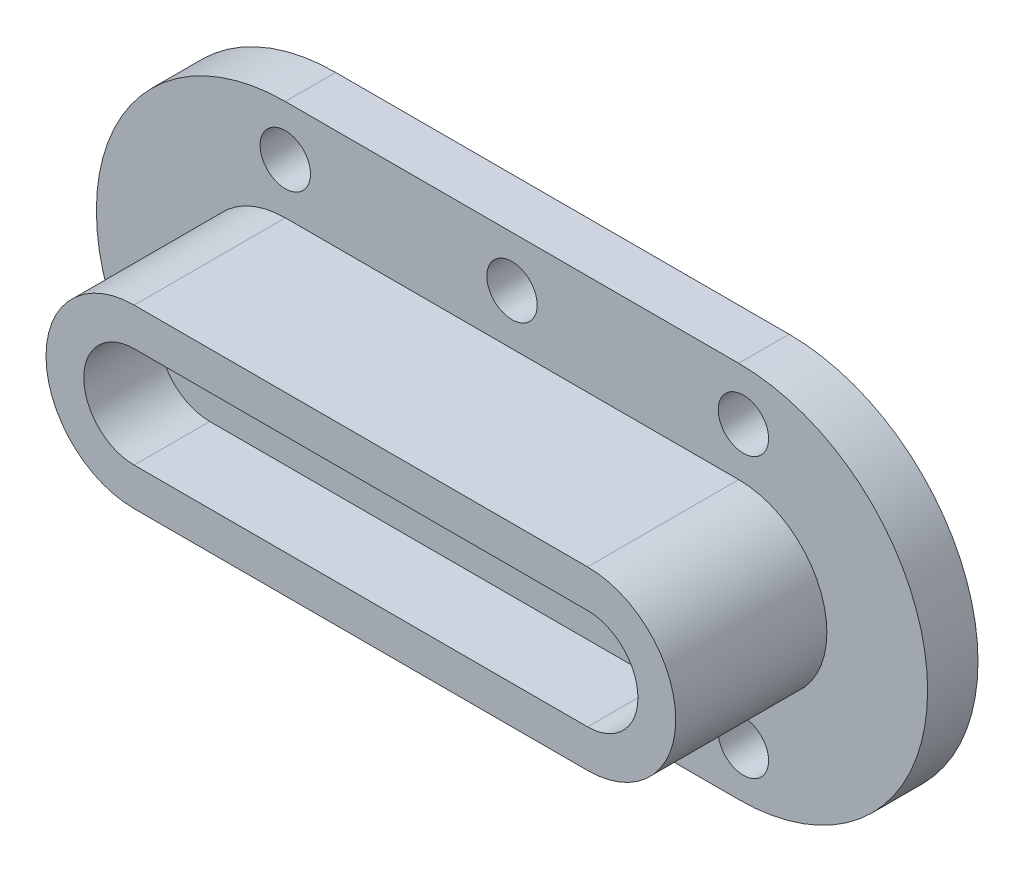
ISO-10303-21;
HEADER;
FILE_DESCRIPTION(('STEP AP214'),'2;1');
FILE_NAME('part.step','',(''),(''),'','','');
FILE_SCHEMA(('AUTOMOTIVE_DESIGN { 1 0 10303 214 1 1 1 1 }'));
ENDSEC;
DATA;
#1=APPLICATION_CONTEXT('core data for automotive mechanical design processes');
#2=APPLICATION_PROTOCOL_DEFINITION('international standard','automotive_design',2000,#1);
#3=PRODUCT_CONTEXT('',#1,'mechanical');
#4=PRODUCT('Part','Part','',(#3));
#5=PRODUCT_RELATED_PRODUCT_CATEGORY('part','',(#4));
#6=PRODUCT_DEFINITION_FORMATION('','',#4);
#7=PRODUCT_DEFINITION_CONTEXT('part definition',#1,'design');
#8=PRODUCT_DEFINITION('design','',#6,#7);
#9=PRODUCT_DEFINITION_SHAPE('','',#8);
#10=(LENGTH_UNIT() NAMED_UNIT(*) SI_UNIT(.MILLI.,.METRE.));
#11=(NAMED_UNIT(*) PLANE_ANGLE_UNIT() SI_UNIT($,.RADIAN.));
#12=(NAMED_UNIT(*) SI_UNIT($,.STERADIAN.) SOLID_ANGLE_UNIT());
#13=UNCERTAINTY_MEASURE_WITH_UNIT(LENGTH_MEASURE(1.E-05),#10,'distance_accuracy_value','');
#14=(GEOMETRIC_REPRESENTATION_CONTEXT(3) GLOBAL_UNCERTAINTY_ASSIGNED_CONTEXT((#13)) GLOBAL_UNIT_ASSIGNED_CONTEXT((#10,
#11,#12)) REPRESENTATION_CONTEXT('',''));
#15=CARTESIAN_POINT('',(0.,0.,0.));
#16=DIRECTION('',(0.,0.,1.));
#17=DIRECTION('',(1.,0.,0.));
#18=AXIS2_PLACEMENT_3D('',#15,#16,#17);
#19=CARTESIAN_POINT('',(0.,0.,20.));
#20=DIRECTION('',(0.,0.,-1.));
#21=DIRECTION('',(-1.,0.,0.));
#22=AXIS2_PLACEMENT_3D('',#19,#20,#21);
#23=CYLINDRICAL_SURFACE('',#22,75.);
#24=CARTESIAN_POINT('',(0.,0.,0.));
#25=DIRECTION('',(0.,0.,1.));
#26=DIRECTION('',(1.,0.,0.));
#27=AXIS2_PLACEMENT_3D('',#24,#25,#26);
#28=CIRCLE('',#27,75.);
#29=CARTESIAN_POINT('',(0.,75.,0.));
#30=VERTEX_POINT('',#29);
#31=CARTESIAN_POINT('',(0.,-75.,0.));
#32=VERTEX_POINT('',#31);
#33=EDGE_CURVE('E202',#30,#32,#28,.T.);
#34=ORIENTED_EDGE('',*,*,#33,.T.);
#35=DIRECTION('',(0.,0.,-1.));
#36=VECTOR('',#35,1.);
#37=CARTESIAN_POINT('',(0.,-75.,20.));
#38=LINE('',#37,#36);
#39=CARTESIAN_POINT('',(0.,-75.,20.));
#40=VERTEX_POINT('',#39);
#41=EDGE_CURVE('E11',#40,#32,#38,.T.);
#42=ORIENTED_EDGE('',*,*,#41,.F.);
#43=CARTESIAN_POINT('',(0.,0.,20.));
#44=DIRECTION('',(0.,0.,1.));
#45=DIRECTION('',(1.,0.,0.));
#46=AXIS2_PLACEMENT_3D('',#43,#44,#45);
#47=CIRCLE('',#46,75.);
#48=CARTESIAN_POINT('',(0.,75.,20.));
#49=VERTEX_POINT('',#48);
#50=EDGE_CURVE('E206',#49,#40,#47,.T.);
#51=ORIENTED_EDGE('',*,*,#50,.F.);
#52=DIRECTION('',(0.,0.,-1.));
#53=VECTOR('',#52,1.);
#54=CARTESIAN_POINT('',(0.,75.,20.));
#55=LINE('',#54,#53);
#56=EDGE_CURVE('E216',#49,#30,#55,.T.);
#57=ORIENTED_EDGE('',*,*,#56,.T.);
#58=EDGE_LOOP('',(#34,#42,#51,#57));
#59=FACE_BOUND('',#58,.T.);
#60=ADVANCED_FACE('F44',(#59),#23,.T.);
#61=CARTESIAN_POINT('',(0.,-75.,20.));
#62=DIRECTION('',(0.,1.,0.));
#63=DIRECTION('',(-1.,0.,0.));
#64=AXIS2_PLACEMENT_3D('',#61,#62,#63);
#65=PLANE('',#64);
#66=DIRECTION('',(1.,0.,0.));
#67=VECTOR('',#66,1.);
#68=CARTESIAN_POINT('',(0.,-75.,0.));
#69=LINE('',#68,#67);
#70=CARTESIAN_POINT('',(180.,-75.,0.));
#71=VERTEX_POINT('',#70);
#72=EDGE_CURVE('E218',#32,#71,#69,.T.);
#73=ORIENTED_EDGE('',*,*,#72,.T.);
#74=DIRECTION('',(0.,0.,-1.));
#75=VECTOR('',#74,1.);
#76=CARTESIAN_POINT('',(180.,-75.,20.));
#77=LINE('',#76,#75);
#78=CARTESIAN_POINT('',(180.,-75.,20.));
#79=VERTEX_POINT('',#78);
#80=EDGE_CURVE('E55',#79,#71,#77,.T.);
#81=ORIENTED_EDGE('',*,*,#80,.F.);
#82=DIRECTION('',(1.,0.,0.));
#83=VECTOR('',#82,1.);
#84=CARTESIAN_POINT('',(0.,-75.,20.));
#85=LINE('',#84,#83);
#86=EDGE_CURVE('E207',#40,#79,#85,.T.);
#87=ORIENTED_EDGE('',*,*,#86,.F.);
#88=ORIENTED_EDGE('',*,*,#41,.T.);
#89=EDGE_LOOP('',(#73,#81,#87,#88));
#90=FACE_BOUND('',#89,.T.);
#91=ADVANCED_FACE('F249',(#90),#65,.F.);
#92=CARTESIAN_POINT('',(180.,0.,20.));
#93=DIRECTION('',(0.,0.,-1.));
#94=DIRECTION('',(-1.,0.,0.));
#95=AXIS2_PLACEMENT_3D('',#92,#93,#94);
#96=CYLINDRICAL_SURFACE('',#95,75.);
#97=CARTESIAN_POINT('',(180.,0.,0.));
#98=DIRECTION('',(0.,0.,1.));
#99=DIRECTION('',(1.,0.,0.));
#100=AXIS2_PLACEMENT_3D('',#97,#98,#99);
#101=CIRCLE('',#100,75.);
#102=CARTESIAN_POINT('',(180.,75.,0.));
#103=VERTEX_POINT('',#102);
#104=EDGE_CURVE('E222',#71,#103,#101,.T.);
#105=ORIENTED_EDGE('',*,*,#104,.T.);
#106=DIRECTION('',(0.,0.,-1.));
#107=VECTOR('',#106,1.);
#108=CARTESIAN_POINT('',(180.,75.,20.));
#109=LINE('',#108,#107);
#110=CARTESIAN_POINT('',(180.,75.,20.));
#111=VERTEX_POINT('',#110);
#112=EDGE_CURVE('E227',#111,#103,#109,.T.);
#113=ORIENTED_EDGE('',*,*,#112,.F.);
#114=CARTESIAN_POINT('',(180.,0.,20.));
#115=DIRECTION('',(0.,0.,1.));
#116=DIRECTION('',(1.,0.,0.));
#117=AXIS2_PLACEMENT_3D('',#114,#115,#116);
#118=CIRCLE('',#117,75.);
#119=EDGE_CURVE('E215',#79,#111,#118,.T.);
#120=ORIENTED_EDGE('',*,*,#119,.F.);
#121=ORIENTED_EDGE('',*,*,#80,.T.);
#122=EDGE_LOOP('',(#105,#113,#120,#121));
#123=FACE_BOUND('',#122,.T.);
#124=ADVANCED_FACE('F231',(#123),#96,.T.);
#125=CARTESIAN_POINT('',(0.,75.,20.));
#126=DIRECTION('',(0.,-1.,0.));
#127=DIRECTION('',(1.,0.,0.));
#128=AXIS2_PLACEMENT_3D('',#125,#126,#127);
#129=PLANE('',#128);
#130=DIRECTION('',(-1.,0.,0.));
#131=VECTOR('',#130,1.);
#132=CARTESIAN_POINT('',(0.,75.,0.));
#133=LINE('',#132,#131);
#134=EDGE_CURVE('E209',#103,#30,#133,.T.);
#135=ORIENTED_EDGE('',*,*,#134,.T.);
#136=ORIENTED_EDGE('',*,*,#56,.F.);
#137=DIRECTION('',(-1.,0.,0.));
#138=VECTOR('',#137,1.);
#139=CARTESIAN_POINT('',(0.,75.,20.));
#140=LINE('',#139,#138);
#141=EDGE_CURVE('E212',#111,#49,#140,.T.);
#142=ORIENTED_EDGE('',*,*,#141,.F.);
#143=ORIENTED_EDGE('',*,*,#112,.T.);
#144=EDGE_LOOP('',(#135,#136,#142,#143));
#145=FACE_BOUND('',#144,.T.);
#146=ADVANCED_FACE('F245',(#145),#129,.F.);
#147=CARTESIAN_POINT('',(0.,0.,20.));
#148=DIRECTION('',(0.,0.,1.));
#149=DIRECTION('',(1.,0.,0.));
#150=AXIS2_PLACEMENT_3D('',#147,#148,#149);
#151=PLANE('',#150);
#152=CARTESIAN_POINT('',(181.871324801107,55.,20.));
#153=DIRECTION('',(0.,0.,1.));
#154=DIRECTION('',(1.,0.,0.));
#155=AXIS2_PLACEMENT_3D('',#152,#153,#154);
#156=CIRCLE('',#155,9.99999999999998);
#157=CARTESIAN_POINT('',(191.871324801107,55.,20.));
#158=VERTEX_POINT('',#157);
#159=EDGE_CURVE('E353',#158,#158,#156,.T.);
#160=ORIENTED_EDGE('',*,*,#159,.F.);
#161=EDGE_LOOP('',(#160));
#162=FACE_BOUND('',#161,.T.);
#163=CARTESIAN_POINT('',(181.871324801107,-55.7131327107115,20.));
#164=DIRECTION('',(0.,0.,1.));
#165=DIRECTION('',(1.,0.,0.));
#166=AXIS2_PLACEMENT_3D('',#163,#164,#165);
#167=CIRCLE('',#166,10.);
#168=CARTESIAN_POINT('',(191.871324801107,-55.7131327107115,20.));
#169=VERTEX_POINT('',#168);
#170=EDGE_CURVE('E359',#169,#169,#167,.T.);
#171=ORIENTED_EDGE('',*,*,#170,.F.);
#172=EDGE_LOOP('',(#171));
#173=FACE_BOUND('',#172,.T.);
#174=CARTESIAN_POINT('',(0.,-55.7131327107115,20.));
#175=DIRECTION('',(0.,0.,1.));
#176=DIRECTION('',(1.,0.,0.));
#177=AXIS2_PLACEMENT_3D('',#174,#175,#176);
#178=CIRCLE('',#177,10.);
#179=CARTESIAN_POINT('',(10.,-55.7131327107115,20.));
#180=VERTEX_POINT('',#179);
#181=EDGE_CURVE('E364',#180,#180,#178,.T.);
#182=ORIENTED_EDGE('',*,*,#181,.F.);
#183=EDGE_LOOP('',(#182));
#184=FACE_BOUND('',#183,.T.);
#185=CARTESIAN_POINT('',(90.,55.,20.));
#186=DIRECTION('',(0.,0.,1.));
#187=DIRECTION('',(1.,0.,0.));
#188=AXIS2_PLACEMENT_3D('',#185,#186,#187);
#189=CIRCLE('',#188,10.);
#190=CARTESIAN_POINT('',(100.,55.,20.));
#191=VERTEX_POINT('',#190);
#192=EDGE_CURVE('E347',#191,#191,#189,.T.);
#193=ORIENTED_EDGE('',*,*,#192,.F.);
#194=EDGE_LOOP('',(#193));
#195=FACE_BOUND('',#194,.T.);
#196=CARTESIAN_POINT('',(90.,-55.7131327107115,20.));
#197=DIRECTION('',(0.,0.,1.));
#198=DIRECTION('',(1.,0.,0.));
#199=AXIS2_PLACEMENT_3D('',#196,#197,#198);
#200=CIRCLE('',#199,9.99999999999999);
#201=CARTESIAN_POINT('',(100.,-55.7131327107115,20.));
#202=VERTEX_POINT('',#201);
#203=EDGE_CURVE('E341',#202,#202,#200,.T.);
#204=ORIENTED_EDGE('',*,*,#203,.F.);
#205=EDGE_LOOP('',(#204));
#206=FACE_BOUND('',#205,.T.);
#207=CARTESIAN_POINT('',(0.,55.,20.));
#208=DIRECTION('',(0.,0.,1.));
#209=DIRECTION('',(1.,0.,0.));
#210=AXIS2_PLACEMENT_3D('',#207,#208,#209);
#211=CIRCLE('',#210,10.);
#212=CARTESIAN_POINT('',(10.,55.,20.));
#213=VERTEX_POINT('',#212);
#214=EDGE_CURVE('E355',#213,#213,#211,.T.);
#215=ORIENTED_EDGE('',*,*,#214,.F.);
#216=EDGE_LOOP('',(#215));
#217=FACE_BOUND('',#216,.T.);
#218=CARTESIAN_POINT('',(0.,0.,20.));
#219=DIRECTION('',(0.,0.,1.));
#220=DIRECTION('',(1.,0.,0.));
#221=AXIS2_PLACEMENT_3D('',#218,#219,#220);
#222=CIRCLE('',#221,35.);
#223=CARTESIAN_POINT('',(0.,35.,20.));
#224=VERTEX_POINT('',#223);
#225=CARTESIAN_POINT('',(0.,-35.,20.));
#226=VERTEX_POINT('',#225);
#227=EDGE_CURVE('E70',#224,#226,#222,.T.);
#228=ORIENTED_EDGE('',*,*,#227,.F.);
#229=DIRECTION('',(-1.,0.,0.));
#230=VECTOR('',#229,1.);
#231=CARTESIAN_POINT('',(0.,35.,20.));
#232=LINE('',#231,#230);
#233=CARTESIAN_POINT('',(180.,35.,20.));
#234=VERTEX_POINT('',#233);
#235=EDGE_CURVE('E179',#234,#224,#232,.T.);
#236=ORIENTED_EDGE('',*,*,#235,.F.);
#237=CARTESIAN_POINT('',(180.,0.,20.));
#238=DIRECTION('',(0.,0.,1.));
#239=DIRECTION('',(1.,0.,0.));
#240=AXIS2_PLACEMENT_3D('',#237,#238,#239);
#241=CIRCLE('',#240,35.);
#242=CARTESIAN_POINT('',(180.,-35.,20.));
#243=VERTEX_POINT('',#242);
#244=EDGE_CURVE('E186',#243,#234,#241,.T.);
#245=ORIENTED_EDGE('',*,*,#244,.F.);
#246=DIRECTION('',(1.,0.,0.));
#247=VECTOR('',#246,1.);
#248=CARTESIAN_POINT('',(0.,-35.,20.));
#249=LINE('',#248,#247);
#250=EDGE_CURVE('E190',#226,#243,#249,.T.);
#251=ORIENTED_EDGE('',*,*,#250,.F.);
#252=EDGE_LOOP('',(#228,#236,#245,#251));
#253=FACE_BOUND('',#252,.T.);
#254=ORIENTED_EDGE('',*,*,#50,.T.);
#255=ORIENTED_EDGE('',*,*,#86,.T.);
#256=ORIENTED_EDGE('',*,*,#119,.T.);
#257=ORIENTED_EDGE('',*,*,#141,.T.);
#258=EDGE_LOOP('',(#254,#255,#256,#257));
#259=FACE_BOUND('',#258,.T.);
#260=ADVANCED_FACE('F246',(#162,#173,#184,#195,#206,#217,#253,#259),#151,.T.);
#261=CARTESIAN_POINT('',(0.,0.,0.));
#262=DIRECTION('',(0.,0.,1.));
#263=DIRECTION('',(1.,0.,0.));
#264=AXIS2_PLACEMENT_3D('',#261,#262,#263);
#265=PLANE('',#264);
#266=CARTESIAN_POINT('',(181.871324801107,55.,0.));
#267=DIRECTION('',(0.,0.,1.));
#268=DIRECTION('',(1.,0.,0.));
#269=AXIS2_PLACEMENT_3D('',#266,#267,#268);
#270=CIRCLE('',#269,9.99999999999998);
#271=CARTESIAN_POINT('',(191.871324801107,55.,0.));
#272=VERTEX_POINT('',#271);
#273=EDGE_CURVE('E349',#272,#272,#270,.T.);
#274=ORIENTED_EDGE('',*,*,#273,.T.);
#275=EDGE_LOOP('',(#274));
#276=FACE_BOUND('',#275,.T.);
#277=CARTESIAN_POINT('',(181.871324801107,-55.7131327107115,0.));
#278=DIRECTION('',(0.,0.,1.));
#279=DIRECTION('',(1.,0.,0.));
#280=AXIS2_PLACEMENT_3D('',#277,#278,#279);
#281=CIRCLE('',#280,10.);
#282=CARTESIAN_POINT('',(191.871324801107,-55.7131327107115,0.));
#283=VERTEX_POINT('',#282);
#284=EDGE_CURVE('E358',#283,#283,#281,.T.);
#285=ORIENTED_EDGE('',*,*,#284,.T.);
#286=EDGE_LOOP('',(#285));
#287=FACE_BOUND('',#286,.T.);
#288=CARTESIAN_POINT('',(0.,-55.7131327107115,0.));
#289=DIRECTION('',(0.,0.,1.));
#290=DIRECTION('',(1.,0.,0.));
#291=AXIS2_PLACEMENT_3D('',#288,#289,#290);
#292=CIRCLE('',#291,10.);
#293=CARTESIAN_POINT('',(10.,-55.7131327107115,0.));
#294=VERTEX_POINT('',#293);
#295=EDGE_CURVE('E362',#294,#294,#292,.T.);
#296=ORIENTED_EDGE('',*,*,#295,.T.);
#297=EDGE_LOOP('',(#296));
#298=FACE_BOUND('',#297,.T.);
#299=CARTESIAN_POINT('',(90.,55.,0.));
#300=DIRECTION('',(0.,0.,1.));
#301=DIRECTION('',(1.,0.,0.));
#302=AXIS2_PLACEMENT_3D('',#299,#300,#301);
#303=CIRCLE('',#302,10.);
#304=CARTESIAN_POINT('',(100.,55.,0.));
#305=VERTEX_POINT('',#304);
#306=EDGE_CURVE('E366',#305,#305,#303,.T.);
#307=ORIENTED_EDGE('',*,*,#306,.T.);
#308=EDGE_LOOP('',(#307));
#309=FACE_BOUND('',#308,.T.);
#310=CARTESIAN_POINT('',(90.,-55.7131327107115,0.));
#311=DIRECTION('',(0.,0.,1.));
#312=DIRECTION('',(1.,0.,0.));
#313=AXIS2_PLACEMENT_3D('',#310,#311,#312);
#314=CIRCLE('',#313,9.99999999999999);
#315=CARTESIAN_POINT('',(100.,-55.7131327107115,0.));
#316=VERTEX_POINT('',#315);
#317=EDGE_CURVE('E336',#316,#316,#314,.T.);
#318=ORIENTED_EDGE('',*,*,#317,.T.);
#319=EDGE_LOOP('',(#318));
#320=FACE_BOUND('',#319,.T.);
#321=CARTESIAN_POINT('',(0.,55.,0.));
#322=DIRECTION('',(0.,0.,1.));
#323=DIRECTION('',(1.,0.,0.));
#324=AXIS2_PLACEMENT_3D('',#321,#322,#323);
#325=CIRCLE('',#324,10.);
#326=CARTESIAN_POINT('',(10.,55.,0.));
#327=VERTEX_POINT('',#326);
#328=EDGE_CURVE('E373',#327,#327,#325,.T.);
#329=ORIENTED_EDGE('',*,*,#328,.T.);
#330=EDGE_LOOP('',(#329));
#331=FACE_BOUND('',#330,.T.);
#332=CARTESIAN_POINT('',(0.,0.,0.));
#333=DIRECTION('',(0.,0.,1.));
#334=DIRECTION('',(1.,0.,0.));
#335=AXIS2_PLACEMENT_3D('',#332,#333,#334);
#336=CIRCLE('',#335,7.5);
#337=CARTESIAN_POINT('',(7.5,0.,0.));
#338=VERTEX_POINT('',#337);
#339=EDGE_CURVE('E167',#338,#338,#336,.T.);
#340=ORIENTED_EDGE('',*,*,#339,.T.);
#341=EDGE_LOOP('',(#340));
#342=FACE_BOUND('',#341,.T.);
#343=CARTESIAN_POINT('',(180.,0.,0.));
#344=DIRECTION('',(0.,0.,1.));
#345=DIRECTION('',(1.,0.,0.));
#346=AXIS2_PLACEMENT_3D('',#343,#344,#345);
#347=CIRCLE('',#346,7.50000000000001);
#348=CARTESIAN_POINT('',(187.5,0.,0.));
#349=VERTEX_POINT('',#348);
#350=EDGE_CURVE('E382',#349,#349,#347,.T.);
#351=ORIENTED_EDGE('',*,*,#350,.T.);
#352=EDGE_LOOP('',(#351));
#353=FACE_BOUND('',#352,.T.);
#354=CARTESIAN_POINT('',(90.,0.,0.));
#355=DIRECTION('',(0.,0.,1.));
#356=DIRECTION('',(1.,0.,0.));
#357=AXIS2_PLACEMENT_3D('',#354,#355,#356);
#358=CIRCLE('',#357,7.5);
#359=CARTESIAN_POINT('',(97.5,0.,0.));
#360=VERTEX_POINT('',#359);
#361=EDGE_CURVE('E389',#360,#360,#358,.T.);
#362=ORIENTED_EDGE('',*,*,#361,.T.);
#363=EDGE_LOOP('',(#362));
#364=FACE_BOUND('',#363,.T.);
#365=ORIENTED_EDGE('',*,*,#33,.F.);
#366=ORIENTED_EDGE('',*,*,#134,.F.);
#367=ORIENTED_EDGE('',*,*,#104,.F.);
#368=ORIENTED_EDGE('',*,*,#72,.F.);
#369=EDGE_LOOP('',(#365,#366,#367,#368));
#370=FACE_BOUND('',#369,.T.);
#371=ADVANCED_FACE('F239',(#276,#287,#298,#309,#320,#331,#342,#353,#364,#370),#265,.F.);
#372=CARTESIAN_POINT('',(0.,0.,80.));
#373=DIRECTION('',(0.,0.,-1.));
#374=DIRECTION('',(-1.,0.,0.));
#375=AXIS2_PLACEMENT_3D('',#372,#373,#374);
#376=CYLINDRICAL_SURFACE('',#375,35.);
#377=ORIENTED_EDGE('',*,*,#227,.T.);
#378=DIRECTION('',(0.,0.,-1.));
#379=VECTOR('',#378,1.);
#380=CARTESIAN_POINT('',(0.,-35.,80.));
#381=LINE('',#380,#379);
#382=CARTESIAN_POINT('',(0.,-35.,80.));
#383=VERTEX_POINT('',#382);
#384=EDGE_CURVE('E205',#383,#226,#381,.T.);
#385=ORIENTED_EDGE('',*,*,#384,.F.);
#386=CARTESIAN_POINT('',(0.,0.,80.));
#387=DIRECTION('',(0.,0.,1.));
#388=DIRECTION('',(1.,0.,0.));
#389=AXIS2_PLACEMENT_3D('',#386,#387,#388);
#390=CIRCLE('',#389,35.);
#391=CARTESIAN_POINT('',(0.,35.,80.));
#392=VERTEX_POINT('',#391);
#393=EDGE_CURVE('E171',#392,#383,#390,.T.);
#394=ORIENTED_EDGE('',*,*,#393,.F.);
#395=DIRECTION('',(0.,0.,-1.));
#396=VECTOR('',#395,1.);
#397=CARTESIAN_POINT('',(0.,35.,80.));
#398=LINE('',#397,#396);
#399=EDGE_CURVE('E183',#392,#224,#398,.T.);
#400=ORIENTED_EDGE('',*,*,#399,.T.);
#401=EDGE_LOOP('',(#377,#385,#394,#400));
#402=FACE_BOUND('',#401,.T.);
#403=ADVANCED_FACE('F261',(#402),#376,.T.);
#404=CARTESIAN_POINT('',(0.,-35.,80.));
#405=DIRECTION('',(0.,1.,0.));
#406=DIRECTION('',(0.,0.,1.));
#407=AXIS2_PLACEMENT_3D('',#404,#405,#406);
#408=PLANE('',#407);
#409=ORIENTED_EDGE('',*,*,#250,.T.);
#410=DIRECTION('',(0.,0.,-1.));
#411=VECTOR('',#410,1.);
#412=CARTESIAN_POINT('',(180.,-35.,80.));
#413=LINE('',#412,#411);
#414=CARTESIAN_POINT('',(180.,-35.,80.));
#415=VERTEX_POINT('',#414);
#416=EDGE_CURVE('E200',#415,#243,#413,.T.);
#417=ORIENTED_EDGE('',*,*,#416,.F.);
#418=DIRECTION('',(1.,0.,0.));
#419=VECTOR('',#418,1.);
#420=CARTESIAN_POINT('',(0.,-35.,80.));
#421=LINE('',#420,#419);
#422=EDGE_CURVE('E176',#383,#415,#421,.T.);
#423=ORIENTED_EDGE('',*,*,#422,.F.);
#424=ORIENTED_EDGE('',*,*,#384,.T.);
#425=EDGE_LOOP('',(#409,#417,#423,#424));
#426=FACE_BOUND('',#425,.T.);
#427=ADVANCED_FACE('F268',(#426),#408,.F.);
#428=CARTESIAN_POINT('',(180.,0.,80.));
#429=DIRECTION('',(0.,0.,-1.));
#430=DIRECTION('',(-1.,0.,0.));
#431=AXIS2_PLACEMENT_3D('',#428,#429,#430);
#432=CYLINDRICAL_SURFACE('',#431,35.);
#433=ORIENTED_EDGE('',*,*,#244,.T.);
#434=DIRECTION('',(0.,0.,-1.));
#435=VECTOR('',#434,1.);
#436=CARTESIAN_POINT('',(180.,35.,80.));
#437=LINE('',#436,#435);
#438=CARTESIAN_POINT('',(180.,35.,80.));
#439=VERTEX_POINT('',#438);
#440=EDGE_CURVE('E198',#439,#234,#437,.T.);
#441=ORIENTED_EDGE('',*,*,#440,.F.);
#442=CARTESIAN_POINT('',(180.,0.,80.));
#443=DIRECTION('',(0.,0.,1.));
#444=DIRECTION('',(1.,0.,0.));
#445=AXIS2_PLACEMENT_3D('',#442,#443,#444);
#446=CIRCLE('',#445,35.);
#447=EDGE_CURVE('E182',#415,#439,#446,.T.);
#448=ORIENTED_EDGE('',*,*,#447,.F.);
#449=ORIENTED_EDGE('',*,*,#416,.T.);
#450=EDGE_LOOP('',(#433,#441,#448,#449));
#451=FACE_BOUND('',#450,.T.);
#452=ADVANCED_FACE('F275',(#451),#432,.T.);
#453=CARTESIAN_POINT('',(0.,35.,80.));
#454=DIRECTION('',(0.,-1.,0.));
#455=DIRECTION('',(0.,0.,-1.));
#456=AXIS2_PLACEMENT_3D('',#453,#454,#455);
#457=PLANE('',#456);
#458=ORIENTED_EDGE('',*,*,#235,.T.);
#459=ORIENTED_EDGE('',*,*,#399,.F.);
#460=DIRECTION('',(-1.,0.,0.));
#461=VECTOR('',#460,1.);
#462=CARTESIAN_POINT('',(0.,35.,80.));
#463=LINE('',#462,#461);
#464=EDGE_CURVE('E181',#439,#392,#463,.T.);
#465=ORIENTED_EDGE('',*,*,#464,.F.);
#466=ORIENTED_EDGE('',*,*,#440,.T.);
#467=EDGE_LOOP('',(#458,#459,#465,#466));
#468=FACE_BOUND('',#467,.T.);
#469=ADVANCED_FACE('F277',(#468),#457,.F.);
#470=CARTESIAN_POINT('',(0.,0.,80.));
#471=DIRECTION('',(0.,0.,1.));
#472=DIRECTION('',(1.,0.,0.));
#473=AXIS2_PLACEMENT_3D('',#470,#471,#472);
#474=PLANE('',#473);
#475=CARTESIAN_POINT('',(0.,0.,80.));
#476=DIRECTION('',(0.,0.,1.));
#477=DIRECTION('',(1.,0.,0.));
#478=AXIS2_PLACEMENT_3D('',#475,#476,#477);
#479=CIRCLE('',#478,20.);
#480=CARTESIAN_POINT('',(0.,20.,80.));
#481=VERTEX_POINT('',#480);
#482=CARTESIAN_POINT('',(0.,-20.,80.));
#483=VERTEX_POINT('',#482);
#484=EDGE_CURVE('E56',#481,#483,#479,.T.);
#485=ORIENTED_EDGE('',*,*,#484,.F.);
#486=DIRECTION('',(-1.,0.,0.));
#487=VECTOR('',#486,1.);
#488=CARTESIAN_POINT('',(0.,20.,80.));
#489=LINE('',#488,#487);
#490=CARTESIAN_POINT('',(180.,20.,80.));
#491=VERTEX_POINT('',#490);
#492=EDGE_CURVE('E153',#491,#481,#489,.T.);
#493=ORIENTED_EDGE('',*,*,#492,.F.);
#494=CARTESIAN_POINT('',(180.,0.,80.));
#495=DIRECTION('',(0.,0.,1.));
#496=DIRECTION('',(1.,0.,0.));
#497=AXIS2_PLACEMENT_3D('',#494,#495,#496);
#498=CIRCLE('',#497,20.);
#499=CARTESIAN_POINT('',(180.,-20.,80.));
#500=VERTEX_POINT('',#499);
#501=EDGE_CURVE('E156',#500,#491,#498,.T.);
#502=ORIENTED_EDGE('',*,*,#501,.F.);
#503=DIRECTION('',(1.,0.,0.));
#504=VECTOR('',#503,1.);
#505=CARTESIAN_POINT('',(0.,-20.,80.));
#506=LINE('',#505,#504);
#507=EDGE_CURVE('E164',#483,#500,#506,.T.);
#508=ORIENTED_EDGE('',*,*,#507,.F.);
#509=EDGE_LOOP('',(#485,#493,#502,#508));
#510=FACE_BOUND('',#509,.T.);
#511=ORIENTED_EDGE('',*,*,#393,.T.);
#512=ORIENTED_EDGE('',*,*,#422,.T.);
#513=ORIENTED_EDGE('',*,*,#447,.T.);
#514=ORIENTED_EDGE('',*,*,#464,.T.);
#515=EDGE_LOOP('',(#511,#512,#513,#514));
#516=FACE_BOUND('',#515,.T.);
#517=ADVANCED_FACE('F278',(#510,#516),#474,.T.);
#518=CARTESIAN_POINT('',(0.,0.,50.));
#519=DIRECTION('',(0.,0.,1.));
#520=DIRECTION('',(1.,0.,0.));
#521=AXIS2_PLACEMENT_3D('',#518,#519,#520);
#522=CYLINDRICAL_SURFACE('',#521,20.);
#523=ORIENTED_EDGE('',*,*,#484,.T.);
#524=DIRECTION('',(0.,0.,1.));
#525=VECTOR('',#524,1.);
#526=CARTESIAN_POINT('',(0.,-20.,50.));
#527=LINE('',#526,#525);
#528=CARTESIAN_POINT('',(0.,-20.,50.));
#529=VERTEX_POINT('',#528);
#530=EDGE_CURVE('E132',#529,#483,#527,.T.);
#531=ORIENTED_EDGE('',*,*,#530,.F.);
#532=CARTESIAN_POINT('',(0.,0.,50.));
#533=DIRECTION('',(0.,0.,1.));
#534=DIRECTION('',(1.,0.,0.));
#535=AXIS2_PLACEMENT_3D('',#532,#533,#534);
#536=CIRCLE('',#535,20.);
#537=CARTESIAN_POINT('',(0.,20.,50.));
#538=VERTEX_POINT('',#537);
#539=EDGE_CURVE('E131',#538,#529,#536,.T.);
#540=ORIENTED_EDGE('',*,*,#539,.F.);
#541=DIRECTION('',(0.,0.,1.));
#542=VECTOR('',#541,1.);
#543=CARTESIAN_POINT('',(0.,20.,50.));
#544=LINE('',#543,#542);
#545=EDGE_CURVE('E168',#538,#481,#544,.T.);
#546=ORIENTED_EDGE('',*,*,#545,.T.);
#547=EDGE_LOOP('',(#523,#531,#540,#546));
#548=FACE_BOUND('',#547,.T.);
#549=ADVANCED_FACE('F133',(#548),#522,.F.);
#550=CARTESIAN_POINT('',(0.,20.,50.));
#551=DIRECTION('',(0.,1.,0.));
#552=DIRECTION('',(-1.,0.,0.));
#553=AXIS2_PLACEMENT_3D('',#550,#551,#552);
#554=PLANE('',#553);
#555=ORIENTED_EDGE('',*,*,#492,.T.);
#556=ORIENTED_EDGE('',*,*,#545,.F.);
#557=DIRECTION('',(-1.,0.,0.));
#558=VECTOR('',#557,1.);
#559=CARTESIAN_POINT('',(0.,20.,50.));
#560=LINE('',#559,#558);
#561=CARTESIAN_POINT('',(180.,20.,50.));
#562=VERTEX_POINT('',#561);
#563=EDGE_CURVE('E143',#562,#538,#560,.T.);
#564=ORIENTED_EDGE('',*,*,#563,.F.);
#565=DIRECTION('',(0.,0.,1.));
#566=VECTOR('',#565,1.);
#567=CARTESIAN_POINT('',(180.,20.,50.));
#568=LINE('',#567,#566);
#569=EDGE_CURVE('E175',#562,#491,#568,.T.);
#570=ORIENTED_EDGE('',*,*,#569,.T.);
#571=EDGE_LOOP('',(#555,#556,#564,#570));
#572=FACE_BOUND('',#571,.T.);
#573=ADVANCED_FACE('F290',(#572),#554,.F.);
#574=CARTESIAN_POINT('',(180.,0.,50.));
#575=DIRECTION('',(0.,0.,1.));
#576=DIRECTION('',(1.,0.,0.));
#577=AXIS2_PLACEMENT_3D('',#574,#575,#576);
#578=CYLINDRICAL_SURFACE('',#577,20.);
#579=ORIENTED_EDGE('',*,*,#501,.T.);
#580=ORIENTED_EDGE('',*,*,#569,.F.);
#581=CARTESIAN_POINT('',(180.,0.,50.));
#582=DIRECTION('',(0.,0.,1.));
#583=DIRECTION('',(1.,0.,0.));
#584=AXIS2_PLACEMENT_3D('',#581,#582,#583);
#585=CIRCLE('',#584,20.);
#586=CARTESIAN_POINT('',(180.,-20.,50.));
#587=VERTEX_POINT('',#586);
#588=EDGE_CURVE('E149',#587,#562,#585,.T.);
#589=ORIENTED_EDGE('',*,*,#588,.F.);
#590=DIRECTION('',(0.,0.,1.));
#591=VECTOR('',#590,1.);
#592=CARTESIAN_POINT('',(180.,-20.,50.));
#593=LINE('',#592,#591);
#594=EDGE_CURVE('E137',#587,#500,#593,.T.);
#595=ORIENTED_EDGE('',*,*,#594,.T.);
#596=EDGE_LOOP('',(#579,#580,#589,#595));
#597=FACE_BOUND('',#596,.T.);
#598=ADVANCED_FACE('F287',(#597),#578,.F.);
#599=CARTESIAN_POINT('',(0.,-20.,50.));
#600=DIRECTION('',(0.,-1.,0.));
#601=DIRECTION('',(1.,0.,0.));
#602=AXIS2_PLACEMENT_3D('',#599,#600,#601);
#603=PLANE('',#602);
#604=ORIENTED_EDGE('',*,*,#507,.T.);
#605=ORIENTED_EDGE('',*,*,#594,.F.);
#606=DIRECTION('',(1.,0.,0.));
#607=VECTOR('',#606,1.);
#608=CARTESIAN_POINT('',(0.,-20.,50.));
#609=LINE('',#608,#607);
#610=EDGE_CURVE('E145',#529,#587,#609,.T.);
#611=ORIENTED_EDGE('',*,*,#610,.F.);
#612=ORIENTED_EDGE('',*,*,#530,.T.);
#613=EDGE_LOOP('',(#604,#605,#611,#612));
#614=FACE_BOUND('',#613,.T.);
#615=ADVANCED_FACE('F144',(#614),#603,.F.);
#616=CARTESIAN_POINT('',(0.,0.,50.));
#617=DIRECTION('',(0.,0.,1.));
#618=DIRECTION('',(1.,0.,0.));
#619=AXIS2_PLACEMENT_3D('',#616,#617,#618);
#620=PLANE('',#619);
#621=CARTESIAN_POINT('',(0.,0.,50.));
#622=DIRECTION('',(0.,0.,1.));
#623=DIRECTION('',(1.,0.,0.));
#624=AXIS2_PLACEMENT_3D('',#621,#622,#623);
#625=CIRCLE('',#624,7.5);
#626=CARTESIAN_POINT('',(7.5,0.,50.));
#627=VERTEX_POINT('',#626);
#628=EDGE_CURVE('E379',#627,#627,#625,.T.);
#629=ORIENTED_EDGE('',*,*,#628,.F.);
#630=EDGE_LOOP('',(#629));
#631=FACE_BOUND('',#630,.T.);
#632=CARTESIAN_POINT('',(180.,0.,50.));
#633=DIRECTION('',(0.,0.,1.));
#634=DIRECTION('',(1.,0.,0.));
#635=AXIS2_PLACEMENT_3D('',#632,#633,#634);
#636=CIRCLE('',#635,7.50000000000001);
#637=CARTESIAN_POINT('',(187.5,0.,50.));
#638=VERTEX_POINT('',#637);
#639=EDGE_CURVE('E387',#638,#638,#636,.T.);
#640=ORIENTED_EDGE('',*,*,#639,.F.);
#641=EDGE_LOOP('',(#640));
#642=FACE_BOUND('',#641,.T.);
#643=CARTESIAN_POINT('',(90.,0.,50.));
#644=DIRECTION('',(0.,0.,1.));
#645=DIRECTION('',(1.,0.,0.));
#646=AXIS2_PLACEMENT_3D('',#643,#644,#645);
#647=CIRCLE('',#646,7.5);
#648=CARTESIAN_POINT('',(97.5,0.,50.));
#649=VERTEX_POINT('',#648);
#650=EDGE_CURVE('E157',#649,#649,#647,.T.);
#651=ORIENTED_EDGE('',*,*,#650,.F.);
#652=EDGE_LOOP('',(#651));
#653=FACE_BOUND('',#652,.T.);
#654=ORIENTED_EDGE('',*,*,#539,.T.);
#655=ORIENTED_EDGE('',*,*,#610,.T.);
#656=ORIENTED_EDGE('',*,*,#588,.T.);
#657=ORIENTED_EDGE('',*,*,#563,.T.);
#658=EDGE_LOOP('',(#654,#655,#656,#657));
#659=FACE_BOUND('',#658,.T.);
#660=ADVANCED_FACE('F151',(#631,#642,#653,#659),#620,.T.);
#661=CARTESIAN_POINT('',(90.,0.,0.));
#662=DIRECTION('',(0.,0.,1.));
#663=DIRECTION('',(1.,0.,0.));
#664=AXIS2_PLACEMENT_3D('',#661,#662,#663);
#665=CYLINDRICAL_SURFACE('',#664,7.5);
#666=ORIENTED_EDGE('',*,*,#361,.F.);
#667=EDGE_LOOP('',(#666));
#668=FACE_BOUND('',#667,.T.);
#669=ORIENTED_EDGE('',*,*,#650,.T.);
#670=EDGE_LOOP('',(#669));
#671=FACE_BOUND('',#670,.T.);
#672=ADVANCED_FACE('F299',(#668,#671),#665,.F.);
#673=CARTESIAN_POINT('',(180.,0.,0.));
#674=DIRECTION('',(0.,0.,1.));
#675=DIRECTION('',(1.,0.,0.));
#676=AXIS2_PLACEMENT_3D('',#673,#674,#675);
#677=CYLINDRICAL_SURFACE('',#676,7.50000000000001);
#678=ORIENTED_EDGE('',*,*,#350,.F.);
#679=EDGE_LOOP('',(#678));
#680=FACE_BOUND('',#679,.T.);
#681=ORIENTED_EDGE('',*,*,#639,.T.);
#682=EDGE_LOOP('',(#681));
#683=FACE_BOUND('',#682,.T.);
#684=ADVANCED_FACE('F301',(#680,#683),#677,.F.);
#685=CARTESIAN_POINT('',(0.,0.,0.));
#686=DIRECTION('',(0.,0.,1.));
#687=DIRECTION('',(1.,0.,0.));
#688=AXIS2_PLACEMENT_3D('',#685,#686,#687);
#689=CYLINDRICAL_SURFACE('',#688,7.5);
#690=ORIENTED_EDGE('',*,*,#339,.F.);
#691=EDGE_LOOP('',(#690));
#692=FACE_BOUND('',#691,.T.);
#693=ORIENTED_EDGE('',*,*,#628,.T.);
#694=EDGE_LOOP('',(#693));
#695=FACE_BOUND('',#694,.T.);
#696=ADVANCED_FACE('F307',(#692,#695),#689,.F.);
#697=CARTESIAN_POINT('',(0.,55.,0.));
#698=DIRECTION('',(0.,0.,1.));
#699=DIRECTION('',(1.,0.,0.));
#700=AXIS2_PLACEMENT_3D('',#697,#698,#699);
#701=CYLINDRICAL_SURFACE('',#700,10.);
#702=ORIENTED_EDGE('',*,*,#328,.F.);
#703=EDGE_LOOP('',(#702));
#704=FACE_BOUND('',#703,.T.);
#705=ORIENTED_EDGE('',*,*,#214,.T.);
#706=EDGE_LOOP('',(#705));
#707=FACE_BOUND('',#706,.T.);
#708=ADVANCED_FACE('F313',(#704,#707),#701,.F.);
#709=CARTESIAN_POINT('',(90.,-55.7131327107115,0.));
#710=DIRECTION('',(0.,0.,1.));
#711=DIRECTION('',(1.,0.,0.));
#712=AXIS2_PLACEMENT_3D('',#709,#710,#711);
#713=CYLINDRICAL_SURFACE('',#712,9.99999999999999);
#714=ORIENTED_EDGE('',*,*,#317,.F.);
#715=EDGE_LOOP('',(#714));
#716=FACE_BOUND('',#715,.T.);
#717=ORIENTED_EDGE('',*,*,#203,.T.);
#718=EDGE_LOOP('',(#717));
#719=FACE_BOUND('',#718,.T.);
#720=ADVANCED_FACE('F312',(#716,#719),#713,.F.);
#721=CARTESIAN_POINT('',(90.,55.,0.));
#722=DIRECTION('',(0.,0.,1.));
#723=DIRECTION('',(1.,0.,0.));
#724=AXIS2_PLACEMENT_3D('',#721,#722,#723);
#725=CYLINDRICAL_SURFACE('',#724,10.);
#726=ORIENTED_EDGE('',*,*,#306,.F.);
#727=EDGE_LOOP('',(#726));
#728=FACE_BOUND('',#727,.T.);
#729=ORIENTED_EDGE('',*,*,#192,.T.);
#730=EDGE_LOOP('',(#729));
#731=FACE_BOUND('',#730,.T.);
#732=ADVANCED_FACE('F320',(#728,#731),#725,.F.);
#733=CARTESIAN_POINT('',(0.,-55.7131327107115,0.));
#734=DIRECTION('',(0.,0.,1.));
#735=DIRECTION('',(1.,0.,0.));
#736=AXIS2_PLACEMENT_3D('',#733,#734,#735);
#737=CYLINDRICAL_SURFACE('',#736,10.);
#738=ORIENTED_EDGE('',*,*,#295,.F.);
#739=EDGE_LOOP('',(#738));
#740=FACE_BOUND('',#739,.T.);
#741=ORIENTED_EDGE('',*,*,#181,.T.);
#742=EDGE_LOOP('',(#741));
#743=FACE_BOUND('',#742,.T.);
#744=ADVANCED_FACE('F319',(#740,#743),#737,.F.);
#745=CARTESIAN_POINT('',(181.871324801107,-55.7131327107115,0.));
#746=DIRECTION('',(0.,0.,1.));
#747=DIRECTION('',(1.,0.,0.));
#748=AXIS2_PLACEMENT_3D('',#745,#746,#747);
#749=CYLINDRICAL_SURFACE('',#748,10.);
#750=ORIENTED_EDGE('',*,*,#284,.F.);
#751=EDGE_LOOP('',(#750));
#752=FACE_BOUND('',#751,.T.);
#753=ORIENTED_EDGE('',*,*,#170,.T.);
#754=EDGE_LOOP('',(#753));
#755=FACE_BOUND('',#754,.T.);
#756=ADVANCED_FACE('F322',(#752,#755),#749,.F.);
#757=CARTESIAN_POINT('',(181.871324801107,55.,0.));
#758=DIRECTION('',(0.,0.,1.));
#759=DIRECTION('',(1.,0.,0.));
#760=AXIS2_PLACEMENT_3D('',#757,#758,#759);
#761=CYLINDRICAL_SURFACE('',#760,9.99999999999998);
#762=ORIENTED_EDGE('',*,*,#273,.F.);
#763=EDGE_LOOP('',(#762));
#764=FACE_BOUND('',#763,.T.);
#765=ORIENTED_EDGE('',*,*,#159,.T.);
#766=EDGE_LOOP('',(#765));
#767=FACE_BOUND('',#766,.T.);
#768=ADVANCED_FACE('F327',(#764,#767),#761,.F.);
#769=CLOSED_SHELL('',(#60,#91,#124,#146,#260,#371,#403,#427,#452,#469,#517,#549,#573,#598,#615,
#660,#672,#684,#696,#708,#720,#732,#744,#756,#768));
#770=MANIFOLD_SOLID_BREP('B2',#769);
#771=ADVANCED_BREP_SHAPE_REPRESENTATION('',(#18,#770),#14);
#772=SHAPE_DEFINITION_REPRESENTATION(#9,#771);
ENDSEC;
END-ISO-10303-21;
